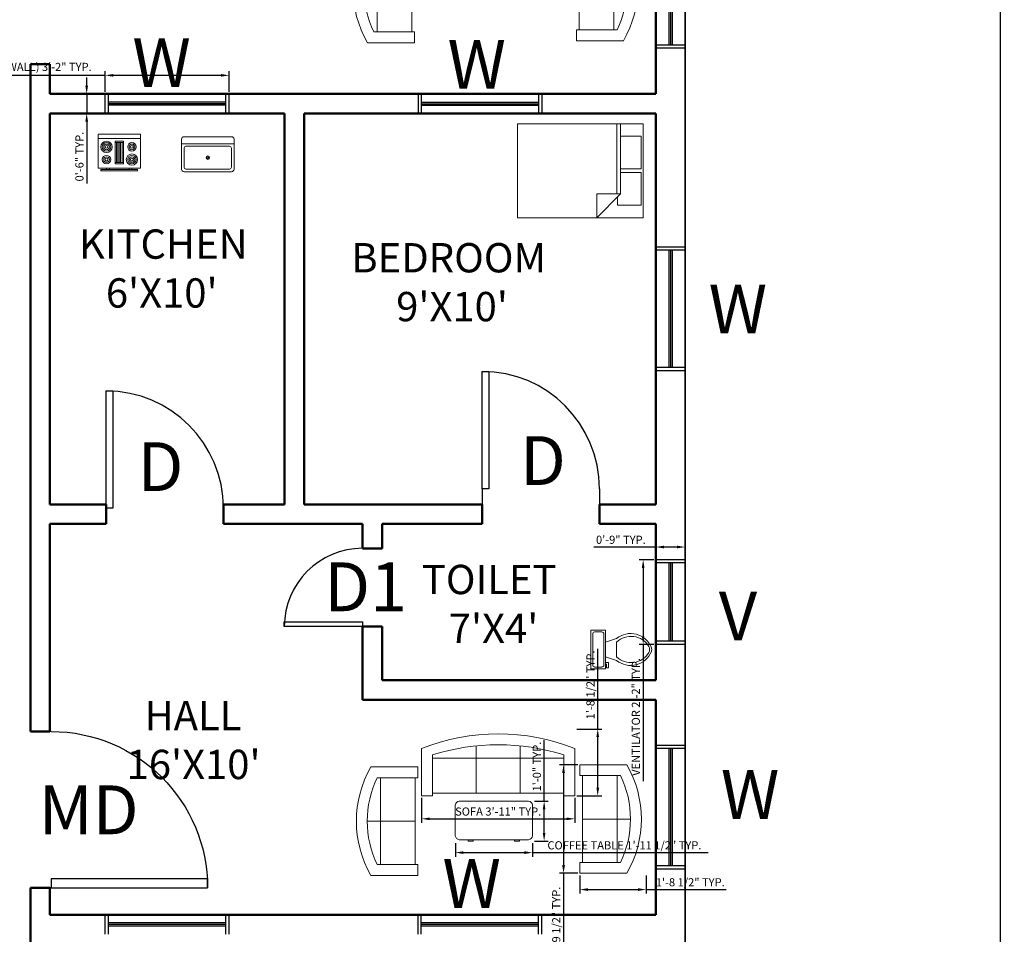
# Model space of a CAD drawing. Units: inches. Extents: x -25308 to -23933, y 10755 to 11996.
# Tile 3 of 6: x -25042 to -24739, y 11402 to 11683. Entities that reach past the tile are written whole.
import ezdxf

# ---------------------------------------------------------------- set-up
doc = ezdxf.new("R2010")
doc.units = ezdxf.units.IN
for name, color, linetype, lineweight in [('A-ANNO-DIMS', 2, 'Continuous', 18), ('A-ANNO-SYMB', 3, 'Continuous', 18), ('A-AREA-IDEN', 7, 'Continuous', 18), ('A-DOOR', 3, 'Continuous', 25), ('A-FLOR-FIXT', 8, 'Continuous', 18), ('A-FURN', 8, 'Continuous', 18), ('A-GLAZ', 4, 'Continuous', 25), ('A-WALL', 7, 'Continuous', 50), ('C-PROP', 30, 'Continuous', 35)]:
    doc.layers.add(name, color=color, linetype=linetype, lineweight=lineweight)
doc.styles.get("Standard").update_dxf_attribs({"font": 'arial.ttf'})
doc.dimstyles.new('ISO-25', dxfattribs={"dimtxt": 2.5, "dimasz": 2.5, "dimexe": 1.25, "dimexo": 0.625, "dimtad": 1, "dimdec": 0, "dimlunit": 3, "dimtxsty": 'Standard', "dimcen": 2.5, "dimadec": 0, "dimazin": 0, "dimtfac": 1, "dimtdec": 0, "dimtmove": 0, "dimatfit": 3, "dimfxl": 1, "dimarcsym": 0})

# ---------------------------------------------------------------- blocks, each defined once
blk = doc.blocks.new('*U8')
for p, q in [((0, 0), (0, -100)), ((750, 0), (750, -100))]:
    blk.add_line(p, q)
blk.add_lwpolyline([(0, 0), (0, 750), (43.75, 750), (43.75, 0)], close=True)
blk.add_arc((0, 0), 750, 0, 90)
blk = doc.blocks.new('Desk - 30 x 60 in.')
for p, q in [((-26.999995, 0), (26.999995, 0)), ((-29.999995, -27), (-29.999995, -3)), ((29.999995, -3), (29.999995, -27)), ((26.999995, -30), (-26.999995, -30)), ((-20.000005, -30), (-20.000005, -31)), ((-16.000005, -31), (-16.000005, -30)), ((15.999995, -31), (15.999995, -30)), ((19.999995, -30), (19.999995, -31)), ((-20.000005, -31), (-16.000005, -31)), ((19.999995, -31), (15.999995, -31))]:
    blk.add_line(p, q)
for centre, start, end in [((-26.499995, -3.5), 98.1301, 171.8699), ((26.499995, -3.5), 8.130102, 81.8699), ((-26.499995, -26.5), 188.1301, 261.8699), ((26.499995, -26.5), 278.1301, 351.8699)]:
    blk.add_arc(centre, 3.535534, start, end)
blk = doc.blocks.new('Sofa - Roundback 7 ft.')
for p, q in [((-12.00002, -32.4421), (-12.00003, -6.5971)), ((11.99997, -32.4421), (11.99998, -6.5971)), ((-36.000027, -34), (-36.000027, -11.4696)), ((-35.999844, -13.3819), (35.9998, -13.3819)), ((35.99998, -34), (35.99998, -11.4696)), ((-36.000027, -32.4421), (35.99998, -32.4421))]:
    blk.add_line(p, q)
for points in [[(-36.000027, -34), (-42.000027, -34), (-42.000027, -8)], [(41.99998, -8), (41.99998, -34), (35.99998, -34)]]:
    blk.add_lwpolyline(points)
for centre, radius, start, end in [((0, -114.25), 114.25, 68.43141, 111.5686), ((-0.00001, -127.1968), 121.1968, 72.72033, 107.2797)]:
    blk.add_arc(centre, radius, start, end)
blk = doc.blocks.new('Sofa - Roundback Loveseat 5 ft.')
for p, q in [((0, -32.44198), (0, -5.99998)), ((-24, -33.99998), (-24, -11.46958)), ((-23.9998, -13.38178), (23.99986, -13.38178)), ((24.00004, -33.99998), (24.00004, -11.46958)), ((-24, -32.44198), (24.00004, -32.44198))]:
    blk.add_line(p, q)
for points in [[(-24, -33.99998), (-30, -33.99998), (-30, -7.99998)], [(30.00004, -7.99998), (30.00004, -33.99998), (24.00004, -33.99998)]]:
    blk.add_lwpolyline(points)
for centre, radius, start, end in [((0, -60.24998), 60.24998, 60.13715, 119.8628), ((0, -61.38438), 55.38444, 64.32083, 115.6792)]:
    blk.add_arc(centre, radius, start, end)
blk = doc.blocks.new('Bed - Queen')
for p, q in [((0, -80.00003), (0, 0)), ((0, 0), (59.99999, 0)), ((59.99999, 0), (59.99999, -80.00003)), ((7.99999, -1.2), (28.79998, -1.2)), ((7.99999, -14.4), (7.99999, -1.2)), ((28.79998, -1.2), (28.79998, -14.4)), ((31.19999, -1.2), (51.99999, -1.2)), ((31.19999, -14.4), (31.19999, -1.2)), ((51.99999, -1.2), (51.99999, -16.4)), ((0, -14.4), (44.8, -14.4)), ((44.8, -16.8), (0, -16.8)), ((59.99999, -29.6), (44.8, -14.4)), ((44.8, -14.4), (44.8, -29.6)), ((51.99999, -16.4), (46.79936, -16.4)), ((44.8, -29.6), (59.99999, -29.6)), ((59.99999, -80.00003), (0, -80.00003))]:
    blk.add_line(p, q)
blk = doc.blocks.new('Range-Oven - 30 in top')
for p, q in [((0, -3), (30, -3)), ((12, -6), (18, -6)), ((13, -20), (13, -6)), ((14, -6), (14, -20)), ((15, -20), (15, -6)), ((16, -6), (16, -20)), ((17, -20), (17, -6)), ((18, -20), (12, -20)), ((6, -24), (6, -25)), ((8, -25), (8, -24)), ((22, -25), (22, -24)), ((24, -24), (24, -25))]:
    blk.add_line(p, q)
for points in [[(0, -24), (0, 0), (30, 0), (30, -24)], [(12, -21), (12, -5), (18, -5), (18, -21)], [(2, -26), (2, -25), (28, -25), (28, -26)]]:
    blk.add_lwpolyline(points, close=True)
for centre, radius in [((6, -9), 4), ((6, -9), 3), ((24, -9), 3), ((6, -9), 2), ((6, -9), 1), ((24, -9), 2), ((24, -9), 1), ((6, -18), 3), ((6, -18), 2), ((6, -18), 1), ((24, -18), 4), ((24, -18), 3), ((24, -18), 2), ((24, -18), 1)]:
    blk.add_circle(centre, radius)
blk = doc.blocks.new('Sink-single - 30 in top')
blk.add_line((-15, -3.999996), (15, -3.999996))
for points in [[(-13.5, 0), (13.5, 0)], [(-15, -18.499996), (-15, -1.5)], [(-12.5, -5.499996), (12.5, -5.499996)], [(15, -1.5), (15, -18.499996)], [(-13.5, -17.499996), (-13.5, -6.499996)], [(13.5, -6.499996), (13.5, -17.499996)], [(13.5, -19.999996), (-13.5, -19.999996)], [(12.5, -18.499996), (-12.5, -18.499996)]]:
    blk.add_lwpolyline(points)
for radius in [1, 0.5]:
    blk.add_circle((0, -11.999996), radius)
for centre, radius, start, end in [((-13.5, -1.5), 1.5, 90, 180), ((-12.5, -6.499996), 1, 90, 180), ((12.5, -6.499996), 1, 0, 90), ((13.5, -1.5), 1.5, 0, 90), ((-13.5, -18.499996), 1.5, 180, 270), ((-12.5, -17.499996), 1, 180, 270), ((12.5, -17.499996), 1, 270, 0), ((13.5, -18.499996), 1.5, 270, 0)]:
    blk.add_arc(centre, radius, start, end)
blk = doc.blocks.new('Toilet - top')
for p, q in [((9.5, -6), (9.5, -2)), ((-10, -8.5), (-8, -8.5)), ((-10, -9.5), (-10, -8.5)), ((-7, -9.5), (-10, -9.5)), ((-8, -8.5), (-8, -8)), ((-7, -8), (-7, -9.5)), ((-4, -8), (-6, -14)), ((4, -8), (6, -14)), ((4, -14), (-4, -14))]:
    blk.add_line(p, q)
blk.add_lwpolyline([(10.5, -8), (10.5, 0), (-10.5, 0), (-10.5, -8)], close=True)
for points in [[(-9.5, -2), (-9.5, -6)], [(8.5, -1), (-8.5, -1)], [(-8.5, -7), (8.5, -7)]]:
    blk.add_lwpolyline(points)
for centre, radius, start, end in [((-8.62, -1.88), 0.884, 81.8699, 188.1301), ((8.62, -1.88), 0.884, 351.8699, 98.1301), ((-8.62, -6.12), 0.884, 171.8699, 278.1301), ((8.62, -6.12), 0.884, 261.8699, 8.1301), ((3.52, -21.58), 12.17, 141.4691, 247.9714), ((4.2, -21.82), 11.33, 136.3677, 238.9468), ((-3.52, -21.58), 12.17, 292.0284, 38.5307), ((-4.2, -21.82), 11.33, 301.053, 43.6321), ((0, -27.88), 4, 245.7318, 294.2682), ((0, -29), 4, 254.8605, 285.1395)]:
    blk.add_arc(centre, radius, start, end)
blk = doc.blocks.new('*D161')
at = {"layer": 'A-ANNO-DIMS', "color": 0, "lineweight": -2, "transparency": 16777216}
for p, q in [((-24836.82, 11915.12), (-24739.49, 11915.12)), ((-24740.74, 11912.62), (-24740.74, 10813.62)), ((-24836.82, 10811.12), (-24739.49, 10811.12))]:
    blk.add_line(p, q, dxfattribs=at)
at = {"layer": 'A-ANNO-DIMS', "color": 0, "transparency": 16777216}
for points in [[(-24741.15, 11912.62), (-24740.32, 11912.62), (-24740.74, 11915.12)], [(-24741.15, 10813.62), (-24740.32, 10813.62), (-24740.74, 10811.12)]]:
    blk.add_solid(points, dxfattribs=at)
at = {"layer": 'Defpoints', "color": 0, "transparency": 16777216}
for p in [(-24837.44, 11915.12), (-24837.44, 10811.12), (-24740.74, 10811.12)]:
    blk.add_point(p, dxfattribs=at)
at = {"layer": 'A-ANNO-DIMS', "color": 0, "transparency": 16777216, "insert": (-24749.53, 11363.12), "char_height": 2.5, "attachment_point": 5, "rotation": 90}
blk.add_mtext("{\\H6.4x;92'}", dxfattribs=at)
blk = doc.blocks.new('WIN-36-9IN')
for p, q in [((0, 9), (0, 0)), ((1, 9), (1, 0)), ((37, 9), (37, 0)), ((38, 9), (38, 0)), ((1, 5), (37, 5)), ((1, 4.5), (37, 4.5)), ((1, 4), (37, 4))]:
    blk.add_line(p, q)
blk = doc.blocks.new('VENT-24')
for p, q in [((0, 26), (9, 26)), ((0, 25), (9, 25)), ((4, 1), (4, 25)), ((4.5, 1), (4.5, 25)), ((5, 1), (5, 25)), ((0, 1), (9, 1)), ((0, 0), (9, 0))]:
    blk.add_line(p, q)
blk = doc.blocks.new('WIN-36-6IN')
for p, q in [((0, 6), (0, 0)), ((1, 6), (1, 0)), ((1, 3.5), (37, 3.5)), ((37, 6), (37, 0)), ((38, 6), (38, 0)), ((1, 3), (37, 3)), ((1, 2.5), (37, 2.5))]:
    blk.add_line(p, q)
blk = doc.blocks.new('*D184')
at = {"layer": 'A-ANNO-DIMS', "color": 0, "lineweight": -2, "transparency": 16777216}
for p, q in [((-25015.44, 11660.75), (-25015.44, 11667.07)), ((-24977.44, 11660.75), (-24977.44, 11667.07)), ((-25015.44, 11665.82), (-25071.37, 11665.82)), ((-24979.94, 11665.82), (-25012.94, 11665.82))]:
    blk.add_line(p, q, dxfattribs=at)
at = {"layer": 'A-ANNO-DIMS', "color": 0, "transparency": 16777216}
for points in [[(-25012.94, 11666.24), (-25012.94, 11665.4), (-25015.44, 11665.82)], [(-24979.94, 11666.24), (-24979.94, 11665.4), (-24977.44, 11665.82)]]:
    blk.add_solid(points, dxfattribs=at)
at = {"layer": 'Defpoints', "color": 0, "transparency": 16777216}
for p in [(-25015.44, 11665.82), (-25015.44, 11660.12), (-24977.44, 11660.12)]:
    blk.add_point(p, dxfattribs=at)
at = {"layer": 'A-ANNO-DIMS', "color": 0, "transparency": 16777216, "insert": (-25044.66, 11668.09), "char_height": 2.5, "attachment_point": 5}
blk.add_mtext('WINDOW 3\' (6" WALL) 3\'-2" TYP.', dxfattribs=at)
blk = doc.blocks.new('*D185')
at = {"layer": 'A-ANNO-DIMS', "color": 0, "lineweight": -2, "transparency": 16777216}
for p, q in [((-25021.14, 11662.62), (-25021.14, 11665.12)), ((-25016.07, 11660.12), (-25022.39, 11660.12)), ((-25021.14, 11660.12), (-25021.14, 11654.12)), ((-25016.07, 11654.12), (-25022.39, 11654.12)), ((-25021.14, 11651.62), (-25021.14, 11632.63))]:
    blk.add_line(p, q, dxfattribs=at)
at = {"layer": 'A-ANNO-DIMS', "color": 0, "transparency": 16777216}
for points in [[(-25021.56, 11662.62), (-25020.73, 11662.62), (-25021.14, 11660.12)], [(-25021.56, 11651.62), (-25020.73, 11651.62), (-25021.14, 11654.12)]]:
    blk.add_solid(points, dxfattribs=at)
at = {"layer": 'Defpoints', "color": 0, "transparency": 16777216}
for p in [(-25015.44, 11660.12), (-25021.14, 11654.12), (-25015.44, 11654.12)]:
    blk.add_point(p, dxfattribs=at)
at = {"layer": 'A-ANNO-DIMS', "color": 0, "transparency": 16777216, "insert": (-25023.05, 11640.88), "char_height": 2.5, "attachment_point": 5, "rotation": 90}
blk.add_mtext('0\'-6" TYP.', dxfattribs=at)
blk = doc.blocks.new('*D188')
at = {"layer": 'A-ANNO-DIMS', "color": 0, "lineweight": -2, "transparency": 16777216}
for p, q in [((-24847.07, 11517.12), (-24851.59, 11517.12)), ((-24850.34, 11514.62), (-24850.34, 11493.62)), ((-24847.07, 11491.12), (-24851.59, 11491.12)), ((-24850.34, 11491.12), (-24850.34, 11449.1))]:
    blk.add_line(p, q, dxfattribs=at)
at = {"layer": 'A-ANNO-DIMS', "color": 0, "transparency": 16777216}
for points in [[(-24850.76, 11514.62), (-24849.93, 11514.62), (-24850.34, 11517.12)], [(-24850.76, 11493.62), (-24849.93, 11493.62), (-24850.34, 11491.12)]]:
    blk.add_solid(points, dxfattribs=at)
at = {"layer": 'Defpoints', "color": 0, "transparency": 16777216}
for p in [(-24846.44, 11517.12), (-24850.34, 11491.12), (-24846.44, 11491.12)]:
    blk.add_point(p, dxfattribs=at)
at = {"layer": 'A-ANNO-DIMS', "color": 0, "transparency": 16777216, "insert": (-24852.26, 11468.86), "char_height": 2.5, "attachment_point": 5, "rotation": 90}
blk.add_mtext('VENTILATOR 2\'-2" TYP.', dxfattribs=at)
blk = doc.blocks.new('*D189')
at = {"layer": 'A-ANNO-DIMS', "color": 0, "lineweight": -2, "transparency": 16777216}
for p, q in [((-24846.44, 11521.02), (-24865.43, 11521.02)), ((-24846.44, 11517.75), (-24846.44, 11522.27)), ((-24839.94, 11521.02), (-24843.94, 11521.02)), ((-24837.44, 11517.75), (-24837.44, 11522.27))]:
    blk.add_line(p, q, dxfattribs=at)
at = {"layer": 'A-ANNO-DIMS', "color": 0, "transparency": 16777216}
for points in [[(-24843.94, 11521.44), (-24843.94, 11520.6), (-24846.44, 11521.02)], [(-24839.94, 11521.44), (-24839.94, 11520.6), (-24837.44, 11521.02)]]:
    blk.add_solid(points, dxfattribs=at)
at = {"layer": 'Defpoints', "color": 0, "transparency": 16777216}
for p in [(-24846.44, 11521.02), (-24846.44, 11517.12), (-24837.44, 11517.12)]:
    blk.add_point(p, dxfattribs=at)
at = {"layer": 'A-ANNO-DIMS', "color": 0, "transparency": 16777216, "insert": (-24857.19, 11522.92), "char_height": 2.5, "attachment_point": 5}
blk.add_mtext('0\'-9" TYP.', dxfattribs=at)
blk = doc.blocks.new('*D190')
at = {"layer": 'A-ANNO-DIMS', "color": 0, "lineweight": -2, "transparency": 16777216}
for p, q in [((-24870.41, 11454.17), (-24876.03, 11454.17)), ((-24874.78, 11451.67), (-24874.78, 11423.35)), ((-24870.41, 11420.85), (-24876.03, 11420.85)), ((-24874.78, 11420.85), (-24874.78, 11376.73))]:
    blk.add_line(p, q, dxfattribs=at)
at = {"layer": 'A-ANNO-DIMS', "color": 0, "transparency": 16777216}
for points in [[(-24875.2, 11451.67), (-24874.36, 11451.67), (-24874.78, 11454.17)], [(-24875.2, 11423.35), (-24874.36, 11423.35), (-24874.78, 11420.85)]]:
    blk.add_solid(points, dxfattribs=at)
at = {"layer": 'Defpoints', "color": 0, "transparency": 16777216}
for p in [(-24869.78, 11454.17), (-24874.78, 11420.85), (-24869.78, 11420.85)]:
    blk.add_point(p, dxfattribs=at)
at = {"layer": 'A-ANNO-DIMS', "color": 0, "transparency": 16777216, "insert": (-24876.7, 11397.54), "char_height": 2.5, "attachment_point": 5, "rotation": 90}
blk.add_mtext('LOVESEAT 2\'-9 1/2" TYP.', dxfattribs=at)
blk = doc.blocks.new('*D191')
at = {"layer": 'A-ANNO-DIMS', "color": 0, "lineweight": -2, "transparency": 16777216}
for p, q in [((-24869.78, 11420.22), (-24869.78, 11414.6)), ((-24849.42, 11420.22), (-24849.42, 11414.6)), ((-24867.28, 11415.85), (-24851.92, 11415.85)), ((-24849.42, 11415.85), (-24824.84, 11415.85))]:
    blk.add_line(p, q, dxfattribs=at)
at = {"layer": 'A-ANNO-DIMS', "color": 0, "transparency": 16777216}
for points in [[(-24867.28, 11416.26), (-24867.28, 11415.43), (-24869.78, 11415.85)], [(-24851.92, 11416.26), (-24851.92, 11415.43), (-24849.42, 11415.85)]]:
    blk.add_solid(points, dxfattribs=at)
at = {"layer": 'Defpoints', "color": 0, "transparency": 16777216}
for p in [(-24869.78, 11420.85), (-24849.42, 11420.85), (-24849.42, 11415.85)]:
    blk.add_point(p, dxfattribs=at)
at = {"layer": 'A-ANNO-DIMS', "color": 0, "transparency": 16777216, "insert": (-24835.88, 11417.77), "char_height": 2.5, "attachment_point": 5}
blk.add_mtext('1\'-8 1/2" TYP.', dxfattribs=at)
blk = doc.blocks.new('*D196')
at = {"layer": 'A-ANNO-DIMS', "color": 0, "lineweight": -2, "transparency": 16777216}
for p, q in [((-24918.35, 11444), (-24918.35, 11436.33)), ((-24871.34, 11444), (-24871.34, 11436.33)), ((-24915.85, 11437.58), (-24873.84, 11437.58))]:
    blk.add_line(p, q, dxfattribs=at)
at = {"layer": 'A-ANNO-DIMS', "color": 0, "transparency": 16777216}
for points in [[(-24915.85, 11437.99), (-24915.85, 11437.16), (-24918.35, 11437.58)], [(-24873.84, 11437.99), (-24873.84, 11437.16), (-24871.34, 11437.58)]]:
    blk.add_solid(points, dxfattribs=at)
at = {"layer": 'Defpoints', "color": 0, "transparency": 16777216}
for p in [(-24918.35, 11444.63), (-24871.34, 11444.63), (-24871.34, 11437.58)]:
    blk.add_point(p, dxfattribs=at)
at = {"layer": 'A-ANNO-DIMS', "color": 0, "transparency": 16777216, "insert": (-24894.84, 11439.49), "char_height": 2.5, "attachment_point": 5}
blk.add_mtext('SOFA 3\'-11" TYP.', dxfattribs=at)
blk = doc.blocks.new('*D197')
at = {"layer": 'A-ANNO-DIMS', "color": 0, "lineweight": -2, "transparency": 16777216}
for p, q in [((-24864.29, 11465.15), (-24864.29, 11489.73)), ((-24870.71, 11465.15), (-24863.04, 11465.15)), ((-24864.29, 11447.13), (-24864.29, 11462.65)), ((-24870.71, 11444.63), (-24863.04, 11444.63))]:
    blk.add_line(p, q, dxfattribs=at)
at = {"layer": 'A-ANNO-DIMS', "color": 0, "transparency": 16777216}
for points in [[(-24864.7, 11462.65), (-24863.87, 11462.65), (-24864.29, 11465.15)], [(-24864.7, 11447.13), (-24863.87, 11447.13), (-24864.29, 11444.63)]]:
    blk.add_solid(points, dxfattribs=at)
at = {"layer": 'Defpoints', "color": 0, "transparency": 16777216}
for p in [(-24871.34, 11465.15), (-24864.29, 11465.15), (-24871.34, 11444.63)]:
    blk.add_point(p, dxfattribs=at)
at = {"layer": 'A-ANNO-DIMS', "color": 0, "transparency": 16777216, "insert": (-24866.2, 11478.69), "char_height": 2.5, "attachment_point": 5, "rotation": 90}
blk.add_mtext('1\'-8 1/2" TYP.', dxfattribs=at)
blk = doc.blocks.new('*D202')
at = {"layer": 'A-ANNO-DIMS', "color": 0, "lineweight": -2, "transparency": 16777216}
for p, q in [((-24907.99, 11430.13), (-24907.99, 11425.95)), ((-24905.49, 11427.2), (-24886.8, 11427.2)), ((-24884.3, 11430.13), (-24884.3, 11425.95)), ((-24884.3, 11427.2), (-24830.4, 11427.2))]:
    blk.add_line(p, q, dxfattribs=at)
at = {"layer": 'A-ANNO-DIMS', "color": 0, "transparency": 16777216}
for points in [[(-24905.49, 11427.62), (-24905.49, 11426.78), (-24907.99, 11427.2)], [(-24886.8, 11427.62), (-24886.8, 11426.78), (-24884.3, 11427.2)]]:
    blk.add_solid(points, dxfattribs=at)
at = {"layer": 'Defpoints', "color": 0, "transparency": 16777216}
for p in [(-24907.99, 11430.75), (-24884.3, 11430.75), (-24884.3, 11427.2)]:
    blk.add_point(p, dxfattribs=at)
at = {"layer": 'A-ANNO-DIMS', "color": 0, "transparency": 16777216, "insert": (-24856.1, 11429.12), "char_height": 2.5, "attachment_point": 5}
blk.add_mtext('COFFEE TABLE 1\'-11 1/2" TYP.', dxfattribs=at)
blk = doc.blocks.new('*D203')
at = {"layer": 'A-ANNO-DIMS', "color": 0, "lineweight": -2, "transparency": 16777216}
for p, q in [((-24880.74, 11443), (-24880.74, 11461.75)), ((-24883.67, 11443), (-24879.49, 11443)), ((-24880.74, 11433.25), (-24880.74, 11440.5)), ((-24883.67, 11430.75), (-24879.49, 11430.75))]:
    blk.add_line(p, q, dxfattribs=at)
at = {"layer": 'A-ANNO-DIMS', "color": 0, "transparency": 16777216}
for points in [[(-24881.16, 11440.5), (-24880.33, 11440.5), (-24880.74, 11443)], [(-24881.16, 11433.25), (-24880.33, 11433.25), (-24880.74, 11430.75)]]:
    blk.add_solid(points, dxfattribs=at)
at = {"layer": 'Defpoints', "color": 0, "transparency": 16777216}
for p in [(-24884.3, 11443), (-24880.74, 11443), (-24884.3, 11430.75)]:
    blk.add_point(p, dxfattribs=at)
at = {"layer": 'A-ANNO-DIMS', "color": 0, "transparency": 16777216, "insert": (-24882.64, 11453.62), "char_height": 2.5, "attachment_point": 5, "rotation": 90}
blk.add_mtext('1\'-0" TYP.', dxfattribs=at)

msp = doc.modelspace()

# ---------------------------------------------------------------- linework, layer by layer
at = {"layer": 'A-WALL'}
for p, q in [((-24846.44, 11726.12), (-24846.44, 11660.12)), ((-25038.44, 11669.22), (-25032.44, 11669.22)), ((-25038.44, 11669.22), (-25038.44, 11464.36)), ((-25032.44, 11669.22), (-25032.44, 11660.12)), ((-25032.44, 11660.12), (-24846.44, 11660.12)), ((-25032.44, 11654.12), (-24960.44, 11654.12)), ((-25032.44, 11654.12), (-25032.44, 11534.12)), ((-24960.44, 11654.12), (-24960.44, 11534.12)), ((-24960.44, 11654.12), (-24960.44, 11534.12)), ((-24960.44, 11654.12), (-24960.44, 11534.12)), ((-24954.44, 11654.12), (-24954.44, 11534.12)), ((-24954.44, 11654.12), (-24954.44, 11534.12)), ((-24954.44, 11654.12), (-24954.44, 11534.12)), ((-24954.44, 11654.12), (-24846.44, 11654.12)), ((-24846.44, 11654.12), (-24846.44, 11534.12)), ((-25032.44, 11534.12), (-25015.18, 11534.12)), ((-25015.18, 11534.12), (-25015.18, 11528.12)), ((-24979.18, 11534.12), (-24979.18, 11528.12)), ((-24979.18, 11534.12), (-24960.44, 11534.12)), ((-24954.44, 11534.12), (-24899.77, 11534.12)), ((-24899.77, 11534.12), (-24899.77, 11528.12)), ((-24863.77, 11534.12), (-24863.77, 11528.12)), ((-24863.77, 11534.12), (-24846.44, 11534.12)), ((-25032.44, 11528.12), (-25015.18, 11528.12)), ((-25032.44, 11528.12), (-25032.44, 11464.36)), ((-24979.18, 11528.12), (-24936.44, 11528.12)), ((-24936.44, 11528.12), (-24936.44, 11520.61)), ((-24936.44, 11528.12), (-24936.44, 11520.61)), ((-24936.44, 11528.12), (-24936.44, 11520.61)), ((-24930.44, 11528.12), (-24930.44, 11520.61)), ((-24930.44, 11528.12), (-24930.44, 11520.61)), ((-24930.44, 11528.12), (-24930.44, 11520.61)), ((-24930.44, 11528.12), (-24899.77, 11528.12)), ((-24863.77, 11528.12), (-24846.44, 11528.12)), ((-24846.44, 11528.12), (-24846.44, 11480.12)), ((-24936.44, 11520.61), (-24930.44, 11520.61)), ((-24936.44, 11496.61), (-24930.44, 11496.61)), ((-24936.44, 11496.61), (-24936.44, 11474.12)), ((-24936.44, 11496.61), (-24936.44, 11474.12)), ((-24936.44, 11496.61), (-24936.44, 11474.12)), ((-24930.44, 11496.61), (-24930.44, 11480.12)), ((-24930.44, 11496.61), (-24930.44, 11480.12)), ((-24930.44, 11496.61), (-24930.44, 11480.12)), ((-24930.44, 11480.12), (-24846.44, 11480.12)), ((-24936.44, 11474.12), (-24846.44, 11474.12)), ((-24846.44, 11474.12), (-24846.44, 11408.12)), ((-25038.44, 11464.36), (-25032.44, 11464.36)), ((-25038.44, 11416.36), (-25032.44, 11416.36)), ((-25038.44, 11416.36), (-25038.44, 11213.64)), ((-25032.44, 11416.36), (-25032.44, 11408.12)), ((-25032.44, 11408.12), (-24846.44, 11408.12))]:
    msp.add_line(p, q, dxfattribs=at)
at = {"layer": 'C-PROP'}
msp.add_line((-24837.44, 11915.12), (-24837.44, 10811.12), dxfattribs=at)

# ---------------------------------------------------------------- block references
at = {"layer": 'A-DOOR', "xscale": 0.0480000000000013, "yscale": 0.0480000000000013, "zscale": 0.0480000000000013}
for p in [(-24899.77, 11538.92), (-25015.18, 11532.92)]:
    msp.add_blockref('*U8', p, dxfattribs=at)
at = {"layer": 'A-DOOR'}
for p, xscale, yscale, zscale, rotation in [((-24936.48, 11496.61), 0.0320095258405211, 0.0320095258405211, 0.0320095258405211, 90), ((-25032.04, 11416.36), -0.0640305237838995, 0.0640305237838995, 0.0640305237838995, 270)]:
    msp.add_blockref('*U8', p, dxfattribs=dict(at, xscale=xscale, yscale=yscale, zscale=zscale, rotation=rotation))
at = {"layer": 'A-FLOR-FIXT'}
for name, p, xscale, yscale, zscale in [('Range-Oven - 30 in top', (-25017.66, 11647.76), 0.4338097128947254, 0.4338097128947254, 0.4338097128947254), ('Sink-single - 30 in top', (-24983.98, 11646.99), 0.5374838416175965, 0.5374838416175965, 0.5374838416175965)]:
    msp.add_blockref(name, p, dxfattribs=dict(at, xscale=xscale, yscale=yscale, zscale=zscale))
at = {"layer": 'A-FLOR-FIXT', "xscale": 0.5659332238665749, "yscale": 0.5659332238665749, "zscale": 0.5659332238665749, "rotation": 90}
msp.add_blockref('Toilet - top', (-24866.4, 11489.56), dxfattribs=at)
at = {"layer": 'A-FURN'}
for name, p, xscale, yscale, zscale, rotation in [('Sofa - Roundback Loveseat 5 ft.', (-24939.4, 11692.47), 0.5553292889469988, 0.5553292889469988, 0.5553292889469988, 89.99999999999999), ('Sofa - Roundback Loveseat 5 ft.', (-24851.93, 11693.12), 0.5553292889469988, 0.5553292889469988, 0.5553292889469988, 270), ('Bed - Queen', (-24850.36, 11650.97), 0.4812808282186369, 0.4812808282186369, 0.4812808282186369, 270), ('Sofa - Roundback Loveseat 5 ft.', (-24938.36, 11436.86), 0.5553292889469988, 0.5553292889469988, 0.5553292889469988, 89.99999999999999), ('Sofa - Roundback Loveseat 5 ft.', (-24850.9, 11437.51), 0.5553292889469988, 0.5553292889469988, 0.5553292889469988, 270)]:
    msp.add_blockref(name, p, dxfattribs=dict(at, xscale=xscale, yscale=yscale, zscale=zscale, rotation=rotation))
for name, p, xscale, yscale, zscale in [('Sofa - Roundback 7 ft.', (-24894.84, 11463.66), 0.559663641165008, 0.559663641165008, 0.559663641165008), ('Desk - 30 x 60 in.', (-24896.15, 11443), 0.3949565101416468, 0.3949565101416468, 0.3949565101416468)]:
    msp.add_blockref(name, p, dxfattribs=dict(at, xscale=xscale, yscale=yscale, zscale=zscale))
at = {"layer": 'A-GLAZ'}
for name, p, rotation in [('WIN-36-9IN', (-24846.44, 11712.12), 270.0000000000173), ('WIN-36-6IN', (-24977.44, 11660.12), 180), ('WIN-36-9IN', (-24846.44, 11613.12), 270.0000000000235), ('VENT-24', (-24837.44, 11517.12), 180), ('VENT-24', (-24837.44, 11517.12), 180), ('WIN-36-9IN', (-24846.44, 11460.12), 270.0000000000211), ('WIN-36-6IN', (-24977.44, 11408.12), 180), ('WIN-36-6IN', (-24881.44, 11408.12), 180)]:
    msp.add_blockref(name, p, dxfattribs=dict(at, rotation=rotation))
msp.add_blockref('WIN-36-6IN', (-24919.44, 11654.12), dxfattribs=at)

# ---------------------------------------------------------------- texts
at = {"layer": 'A-ANNO-SYMB', "char_height": 15, "attachment_point": 1}
for s, insert in [('{W}', (-25007.14, 11677.21)), ('{W}', (-24910.4, 11676.71)), ('{W}', (-24830.25, 11601.57)), ('{D}', (-24888.15, 11555.05)), ('{D}', (-25005.53, 11553.19)), ('{D1}', (-24948.23, 11516.3)), ('{V}', (-24827.12, 11507.33)), ('{W}', (-24826.5, 11452.56)), ('{MD}', (-25035.9, 11447.84)), ('{W}', (-24911.95, 11425.21))]:
    msp.add_mtext_dynamic_manual_height_columns(s, width=1123.2502, gutter_width=12.5, heights=[0], dxfattribs=dict(at, insert=insert))
at = {"layer": 'A-AREA-IDEN', "char_height": 9, "attachment_point": 1}
for s, insert in [("{KITCHEN\\P   6'X10'}", (-25023.51, 11618.52)), ("{BEDROOM\\P     9'X10'}", (-24939.9, 11614.33)), ("{TOILET\\P   7'X4'}", (-24918.26, 11515.55)), ("{     HALL\\P   16'X10'}", (-25017.14, 11473.77))]:
    msp.add_mtext_dynamic_manual_height_columns(s, width=1489.8169, gutter_width=12.5, heights=[0], dxfattribs=dict(at, insert=insert))

# ---------------------------------------------------------------- dimensions: what is measured, and where the dimension line sits
at = {"layer": 'A-ANNO-DIMS'}
for base, p1, p2, angle, text, override, picture, middle in [((-24740.74, 10811.12), (-24837.44, 11915.12), (-24837.44, 10811.12), 90, '{\\H6.4x;<>}', {"dimclrd": 0, "dimclre": 0, "dimclrt": 0}, '*D161', (-24749.53, 11363.12)), ((-25015.44, 11665.82), (-24977.44, 11660.12), (-25015.44, 11660.12), 180, 'WINDOW 3\' (6" WALL) <> TYP.', {"dimdec": 1, "dimlfac": 1, "dimrnd": 0, "dimzin": 1, "dimdsep": 46, "dimlunit": 4, "dimfrac": 2}, '*D184', (-25044.66, 11668.09)), ((-25021.14, 11654.12), (-25015.44, 11660.12), (-25015.44, 11654.12), 270, '<> TYP.', {"dimdec": 1, "dimlfac": 1, "dimrnd": 0, "dimzin": 1, "dimdsep": 46, "dimlunit": 4, "dimfrac": 2}, '*D185', (-25023.05, 11640.88)), ((-24846.44, 11521.02), (-24837.44, 11517.12), (-24846.44, 11517.12), 180, '<> TYP.', {"dimdec": 1, "dimlfac": 1, "dimrnd": 0, "dimzin": 1, "dimdsep": 46, "dimlunit": 4, "dimfrac": 2}, '*D189', (-24857.19, 11522.92)), ((-24850.34, 11491.12), (-24846.44, 11517.12), (-24846.44, 11491.12), 270, 'VENTILATOR <> TYP.', {"dimdec": 1, "dimlfac": 1, "dimrnd": 0, "dimzin": 1, "dimdsep": 46, "dimlunit": 4, "dimfrac": 2}, '*D188', (-24852.26, 11468.86)), ((-24864.29, 11465.15), (-24871.34, 11444.63), (-24871.34, 11465.15), 90, '<> TYP.', {"dimdec": 1, "dimlfac": 1, "dimrnd": 0, "dimzin": 1, "dimdsep": 46, "dimlunit": 4, "dimfrac": 2}, '*D197', (-24866.2, 11478.69)), ((-24880.742, 11442.998), (-24884.2966, 11430.7544), (-24884.2966, 11442.998), 90, '<> TYP.', {"dimdec": 1, "dimlfac": 1, "dimrnd": 0, "dimzin": 1, "dimdsep": 46, "dimlunit": 4, "dimfrac": 2}, '*D203', (-24882.6435, 11453.6247)), ((-24874.78, 11420.85), (-24869.78, 11454.17), (-24869.78, 11420.85), 270, 'LOVESEAT <> TYP.', {"dimdec": 1, "dimlfac": 1, "dimrnd": 0, "dimzin": 1, "dimdsep": 46, "dimlunit": 4, "dimfrac": 2}, '*D190', (-24876.7, 11397.54))]:
    dim = msp.add_linear_dim(base=base, p1=p1, p2=p2, angle=angle, text=text, dimstyle='ISO-25', override=override, dxfattribs=at)
    dim.commit()
    dim.dimension.update_dxf_attribs({"geometry": picture, "text_midpoint": middle})
for base, p1, p2, text, picture, middle in [((-24871.34, 11437.58), (-24918.35, 11444.63), (-24871.34, 11444.63), 'SOFA <> TYP.', '*D196', (-24894.84, 11439.49)), ((-24884.3, 11427.2), (-24907.99, 11430.75), (-24884.3, 11430.75), 'COFFEE TABLE <> TYP.', '*D202', (-24856.1, 11429.12)), ((-24849.42, 11415.85), (-24869.78, 11420.85), (-24849.42, 11420.85), '<> TYP.', '*D191', (-24835.88, 11417.77))]:
    dim = msp.add_linear_dim(base=base, p1=p1, p2=p2, text=text, dimstyle='ISO-25', override={"dimdec": 1, "dimlfac": 1, "dimrnd": 0, "dimzin": 1, "dimdsep": 46, "dimlunit": 4, "dimfrac": 2}, dxfattribs=at)
    dim.commit()
    dim.dimension.update_dxf_attribs({"geometry": picture, "text_midpoint": middle})

doc.saveas('drawing.dxf')
